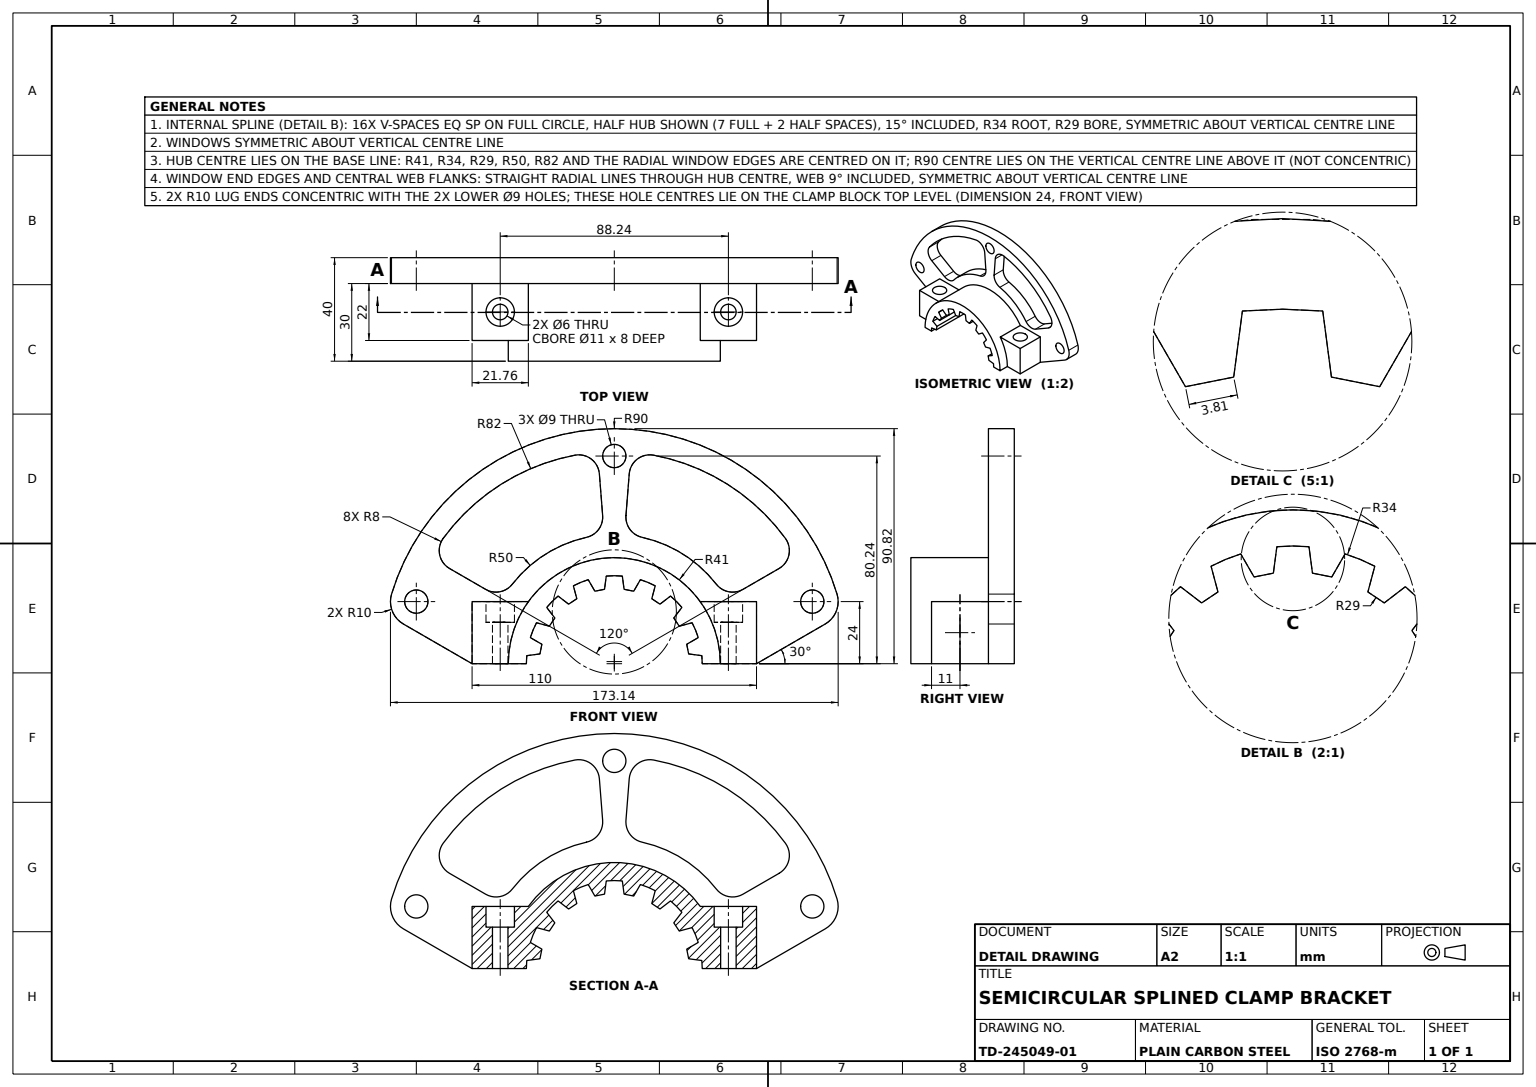
from build123d import *

# Parameters (mm, degrees)
SECTOR_PLATE_SKETCH_R          = 4.5
SECTOR_PLATE_DEPTH             = 10
MOUNTING_LUG_SKETCH_W          = 110
MOUNTING_LUG_SKETCH_H          = 24
MOUNTING_LUGS_DEPTH            = 22
HALF_HUB_DEPTH                 = 30
LUG_C_BORE_HOLES_6_D           = 6
LUG_C_BORE_HOLES_6_DEPTH       = 99.968745116
LUG_C_BORE_HOLES_6_CBORE_D     = 11
LUG_C_BORE_HOLES_6_CBORE_DEPTH = 8
INTERNAL_SPLINE_CUT_DEPTH      = 132.69328114


with BuildPart() as part:
    # Sector Plate Sketch → Sector Plate (new body)
    with BuildSketch(Plane.XY):
        with BuildLine():
            Line((0, 0), (55, 0))
            Line((55, 0), (81.569219382, 15.339745962))
            ThreePointArc((81.569219382, 15.339745962), (85.868282889, 20.322036175), (86.140371804, 26.897074611))
            ThreePointArc((86.140371804, 26.897074611), (0, 90.823403113), (-86.140371804, 26.897074611))
            ThreePointArc((-86.140371804, 26.897074611), (-85.868282889, 20.322036175), (-81.569219382, 15.339745962))
            Line((-81.569219382, 15.339745962), (-55, 0))
            Line((-55, 0), (0, 0))
        make_face()
        with Locations((-76.569219382, 24)):
            Circle(SECTOR_PLATE_SKETCH_R, mode=Mode.SUBTRACT)
        with Locations((76.569219382, 24)):
            Circle(SECTOR_PLATE_SKETCH_R, mode=Mode.SUBTRACT)
        with Locations((0, 80.242416194)):
            Circle(SECTOR_PLATE_SKETCH_R, mode=Mode.SUBTRACT)
        with BuildLine():
            Line((4.507131906, 57.26854077), (5.77194511, 73.33951629))
            ThreePointArc((5.77194511, 73.33951629), (8.888624682, 79.067426249), (15.233476621, 80.572583365))
            ThreePointArc((15.233476621, 80.572583365), (43.756390305, 69.34968138), (66.165447339, 48.436903064))
            ThreePointArc((66.165447339, 48.436903064), (67.538443843, 42.062146233), (63.710281745, 36.783148315))
            Line((63.710281745, 36.783148315), (49.749371855, 28.722813233))
            ThreePointArc((49.749371855, 28.722813233), (44.217975712, 27.798957762), (39.439113668, 30.733634882))
            ThreePointArc((39.439113668, 30.733634882), (26.680725796, 42.286391085), (10.760750496, 48.828334487))
            ThreePointArc((10.760750496, 48.828334487), (6.054600974, 51.878253977), (4.507131906, 57.26854077))
        make_face(mode=Mode.SUBTRACT)
        with BuildLine():
            Line((-4.507131906, 57.26854077), (-5.77194511, 73.33951629))
            ThreePointArc((-5.77194511, 73.33951629), (-8.888624682, 79.067426249), (-15.233476621, 80.572583365))
            ThreePointArc((-15.233476621, 80.572583365), (-43.756390305, 69.34968138), (-66.165447339, 48.436903064))
            ThreePointArc((-66.165447339, 48.436903064), (-67.538443843, 42.062146233), (-63.710281745, 36.783148315))
            Line((-63.710281745, 36.783148315), (-49.749371855, 28.722813233))
            ThreePointArc((-49.749371855, 28.722813233), (-44.217975712, 27.798957762), (-39.439113668, 30.733634882))
            ThreePointArc((-39.439113668, 30.733634882), (-26.680725796, 42.286391085), (-10.760750496, 48.828334487))
            ThreePointArc((-10.760750496, 48.828334487), (-6.054600974, 51.878253977), (-4.507131906, 57.26854077))
        make_face(mode=Mode.SUBTRACT)
    extrude(amount=SECTOR_PLATE_DEPTH)

    # Mounting Lug Sketch → Mounting Lugs (add)
    with BuildSketch(Plane.XY.offset(10)):
        with Locations((0, 12)):
            Rectangle(MOUNTING_LUG_SKETCH_W, MOUNTING_LUG_SKETCH_H)
    extrude(amount=MOUNTING_LUGS_DEPTH)

    # Half Hub Sketch → Half Hub (add)
    with BuildSketch(Plane.XY.offset(10)):
        with BuildLine():
            Line((-41, 0), (41, 0))
            ThreePointArc((41, 0), (0, 41), (-41, 0))
        make_face()
    extrude(amount=HALF_HUB_DEPTH)

    # Lug C'Bore Holes Ø6
    with Locations(Plane(origin=(-44.120770139, 24, 21), x_dir=(0, 0, 1), z_dir=(0, 1, 0))):
        with Locations((0, 0), (0, 88.241540278)):
            CounterBoreHole(LUG_C_BORE_HOLES_6_D / 2, LUG_C_BORE_HOLES_6_CBORE_D / 2, LUG_C_BORE_HOLES_6_CBORE_DEPTH, depth=LUG_C_BORE_HOLES_6_DEPTH)

    # Internal Spline Sketch → Internal Spline Cut (cut, through all)
    with BuildSketch(Plane.XY.offset(40)):
        with BuildLine():
            ThreePointArc((3.107264378, 33.857715636), (0, 34), (-3.107264378, 33.857715636))
            Line((-3.107264378, 33.857715636), (-3.779355377, 28.752677665))
            ThreePointArc((-3.779355377, 28.752677665), (-5.657619338, 28.442773132), (-7.511504299, 28.010307088))
            Line((-7.511504299, 28.010307088), (-10.08604887, 32.469549091))
            ThreePointArc((-10.08604887, 32.469549091), (-13.0112367, 31.411904105), (-15.827524793, 30.091351896))
            Line((-15.827524793, 30.091351896), (-14.494842458, 25.117713712))
            ThreePointArc((-14.494842458, 25.117713712), (-16.111536758, 24.112618757), (-17.658805539, 23.00362117))
            Line((-17.658805539, 23.00362117), (-21.743852609, 26.138188034))
            ThreePointArc((-21.743852609, 26.138188034), (-24.04163056, 24.04163056), (-26.138188034, 21.743852609))
            Line((-26.138188034, 21.743852609), (-23.00362117, 17.658805539))
            ThreePointArc((-23.00362117, 17.658805539), (-24.112618757, 16.111536758), (-25.117713712, 14.494842458))
            Line((-25.117713712, 14.494842458), (-30.091351896, 15.827524793))
            ThreePointArc((-30.091351896, 15.827524793), (-31.411904105, 13.0112367), (-32.469549091, 10.08604887))
            Line((-32.469549091, 10.08604887), (-28.010307088, 7.511504299))
            ThreePointArc((-28.010307088, 7.511504299), (-28.442773132, 5.657619338), (-28.752677665, 3.779355377))
            Line((-28.752677665, 3.779355377), (-33.857715636, 3.107264378))
            ThreePointArc((-33.857715636, 3.107264378), (-33.964410282, 1.555260168), (-34, 0))
            Line((-34, 0), (34, 0))
            ThreePointArc((34, 0), (33.964410282, 1.555260168), (33.857715636, 3.107264378))
            Line((33.857715636, 3.107264378), (28.752677665, 3.779355377))
            ThreePointArc((28.752677665, 3.779355377), (28.442773132, 5.657619338), (28.010307088, 7.511504299))
            Line((28.010307088, 7.511504299), (32.469549091, 10.08604887))
            ThreePointArc((32.469549091, 10.08604887), (31.411904105, 13.0112367), (30.091351896, 15.827524793))
            Line((30.091351896, 15.827524793), (25.117713712, 14.494842458))
            ThreePointArc((25.117713712, 14.494842458), (24.112618757, 16.111536758), (23.00362117, 17.658805539))
            Line((23.00362117, 17.658805539), (26.138188034, 21.743852609))
            ThreePointArc((26.138188034, 21.743852609), (24.04163056, 24.04163056), (21.743852609, 26.138188034))
            Line((21.743852609, 26.138188034), (17.658805539, 23.00362117))
            ThreePointArc((17.658805539, 23.00362117), (16.111536758, 24.112618757), (14.494842458, 25.117713712))
            Line((14.494842458, 25.117713712), (15.827524793, 30.091351896))
            ThreePointArc((15.827524793, 30.091351896), (13.0112367, 31.411904105), (10.08604887, 32.469549091))
            Line((10.08604887, 32.469549091), (7.511504299, 28.010307088))
            ThreePointArc((7.511504299, 28.010307088), (5.657619338, 28.442773132), (3.779355377, 28.752677665))
            Line((3.779355377, 28.752677665), (3.107264378, 33.857715636))
        make_face()
    extrude(amount=-INTERNAL_SPLINE_CUT_DEPTH, mode=Mode.SUBTRACT)


solid = part.part
